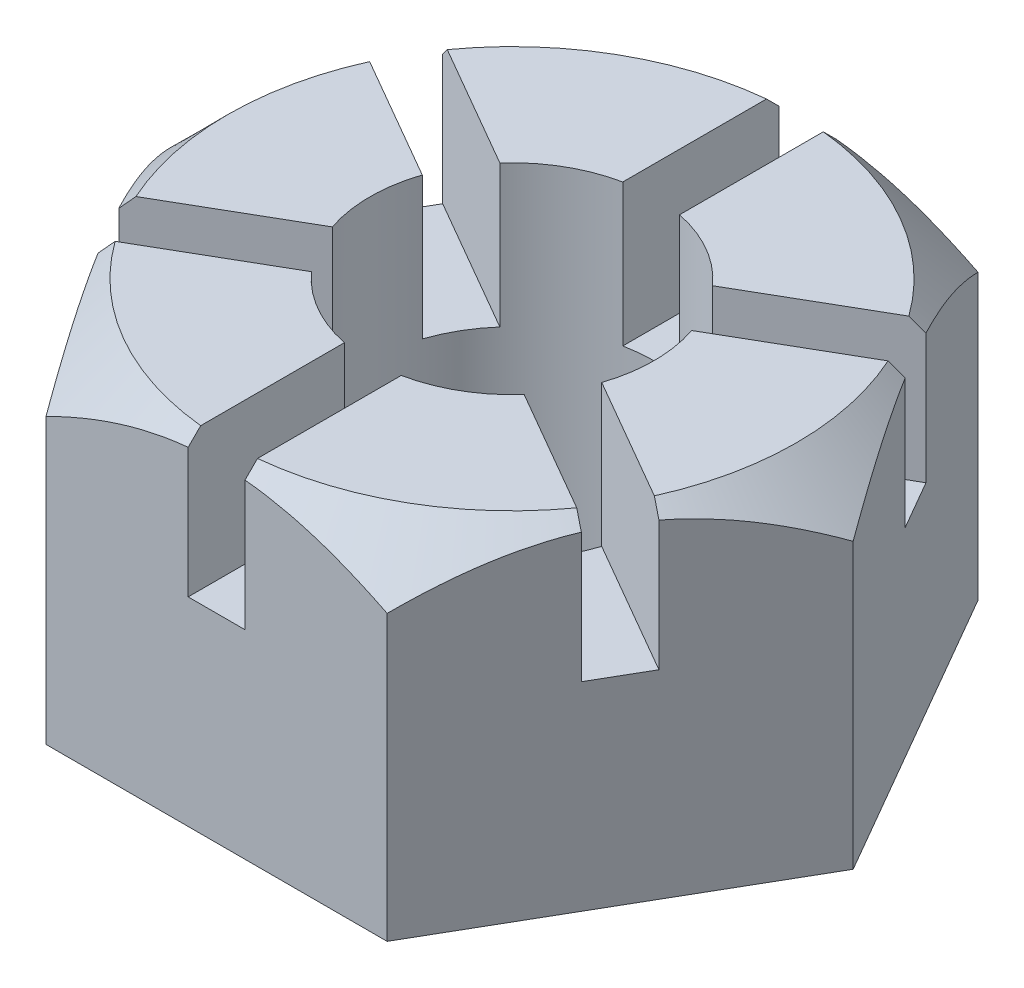
SolidWorks part; units mm, degrees
material "Zinc AC43A (Zn-4Al-2.5Cu-0.04Mg; Number 2 Die Casting Alloy; Zamak 2), Die Cast"
ref_plane "Front Plane" through (0, 0, 0) normal (0, 0, 1) x (1, 0, 0)
ref_plane "Top Plane" through (0, 0, 0) normal (0, 1, 0) x (1, 0, 0)
ref_plane "Right Plane" through (0, 0, 0) normal (1, 0, 0) x (0, 0, -1)
sketch "Hex Profile" plane through (0, 0, 0) normal (0, 1, 0) x (1, 0, 0)
  line L1 (60.0444, 0) -> (30.0222, 52)
  line L2 (30.0222, 52) -> (-30.0222, 52)
  line L3 (-30.0222, 52) -> (-60.0444, 0)
  line L4 (-60.0444, 0) -> (-30.0222, -52)
  line L5 (-30.0222, -52) -> (30.0222, -52)
  line L6 (30.0222, -52) -> (60.0444, 0)
  circle A0 centre (0, 0) radius 52 construction
  circle A1 centre (0, 0) radius 25
  dimension "D2" = 50
  dimension "D1" = 104
extrude "Hex Nut Body" add sketch "Hex Profile" against normal blind 60
sketch "Top Chamfer Profile" plane through (0, 0, 0) normal (0, 0, 1) x (1, 0, 0)
  line L0 (50.0444, 0) -> (60.0444, -10)
  line L1 (60.0444, -60) -> (60.0444, 0) construction
  line L2 (30.0222, 0) -> (60.0444, 0) construction
  line L3 (50.0444, 0) -> (60.0444, 0)
  line L4 (60.0444, 0) -> (60.0444, -10)
  dimension "D1" = 10
  dimension "D2" = 10
revolve "Top Chamfer 10x10" cut sketch "Top Chamfer Profile" angle 360 about axis through (0, -60, 0) along (0, 1, 0)
sketch "Castellation Slot Profile" plane through (0, 0, 0) normal (0, 1, 0) x (1, 0, 0)
  line L0 (30.0222, 52) -> (-30.0222, 52) construction
  line L2 (-5, 24.4949) -> (-5, 52)
  line L3 (-5, 52) -> (5, 52)
  line L4 (5, 24.4949) -> (5, 52)
  circle A0 centre (0, 0) radius 25 construction
  arc A1 (5, 24.4949) -> (-5, 24.4949) centre (0, 0) ccw
  point P9 (0, 52)
  dimension "D1" = 10
extrude "Castellation Slot 10 Wide" cut sketch "Castellation Slot Profile" against normal blind 25
pattern_circular "Castellation Slot Pattern 6x" count 6 over 360 about axis through (0, 0, 0) along (0, 1, 0) of "Castellation Slot 10 Wide"
